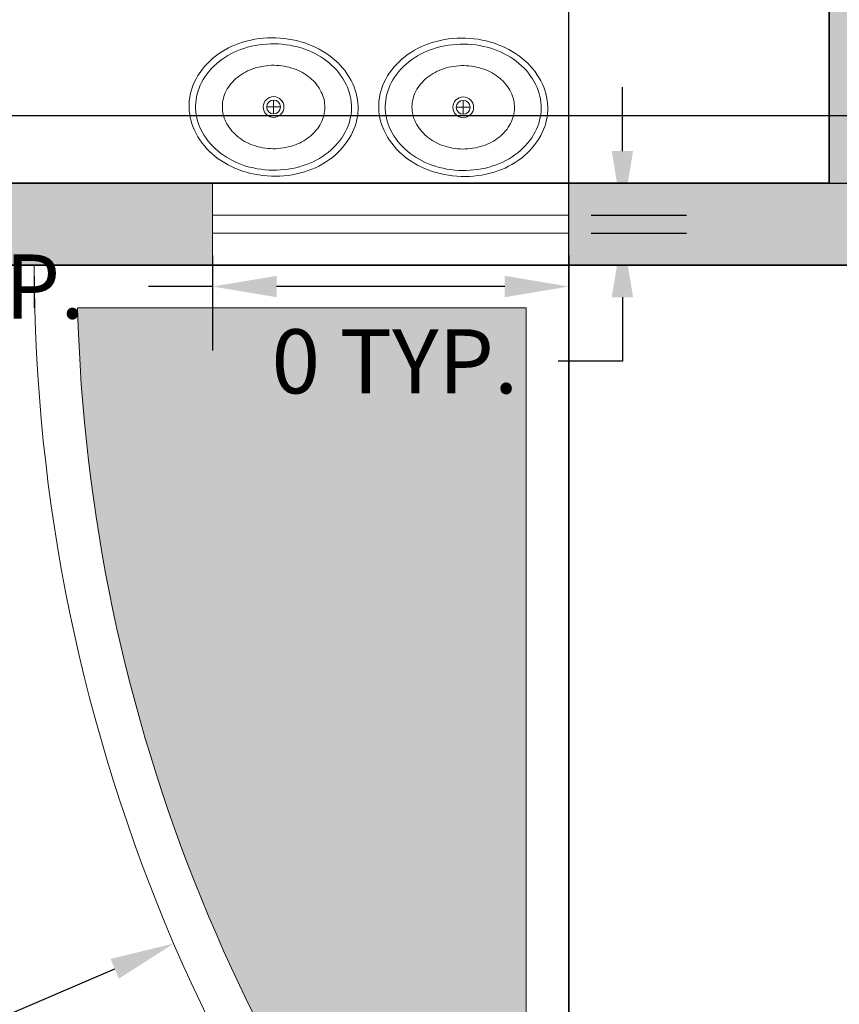
# Model space of a CAD drawing. Units: metres. Extents: x 4298.5 to 4325.2, y 2075 to 2095.8.
# Tile 11 of 35: x 4307.6 to 4309.9, y 2077.8 to 2080.5. Entities that reach past the tile are written whole.
import ezdxf

# ---------------------------------------------------------------- set-up
doc = ezdxf.new("R2010")
doc.units = ezdxf.units.M
for name, color, linetype, lineweight in [('A-ANNO-DIMS', 2, 'Continuous', 18), ('A-FLOR-FIXT', 15, 'Continuous', 18), ('A-FLOR-STRS', 7, 'Continuous', 25), ('A-GLAZ', 4, 'Continuous', 18), ('A-WALL', 7, 'Continuous', 35), ('A-WALL-PATT', 252, 'Continuous', 13), ('L-PLNT-BEDS', 94, 'Continuous', 18), ('L-PLNT-BEDS-PATT', 252, 'Continuous', 13)]:
    doc.layers.add(name, color=color, linetype=linetype, lineweight=lineweight)
doc.styles.get("Standard").update_dxf_attribs({"font": 'arial.ttf'})
doc.dimstyles.get("Standard").update_dxf_attribs({"dimtxt": 0.18, "dimasz": 0.18, "dimexe": 0.18, "dimexo": 0.0625, "dimgap": 0.09, "dimtad": 0, "dimtih": 1, "dimtoh": 1, "dimdec": 4, "dimzin": 0, "dimdsep": 46, "dimtxsty": 'Standard', "dimcen": 0.09, "dimadec": 0, "dimazin": 0, "dimtfac": 1, "dimtdec": 4, "dimtofl": 0, "dimtmove": 0, "dimatfit": 3, "dimfxl": 1, "dimtolj": 1, "dimtzin": 0, "dimarcsym": 0})

# ---------------------------------------------------------------- blocks, each defined once
blk = doc.blocks.new('Sink - Oval top')
for p, q in [((-1, 0), (1, 0)), ((0, 1), (0, -1))]:
    blk.add_line(p, q)
for points in [[(-12.23, 0.39, 0.117634), (-11.46, -3.36, 0.104469), (-8.88, -6.8, 0.090016), (-5.08, -9.07, 0.08192), (-0.32, -10.02, 0.08192), (4.49, -9.38, 0.090016), (8.42, -7.36, 0.104469), (11.22, -4.09, 0.117634), (12.23, -0.39, 0.117634), (11.46, 3.36, 0.104469), (8.88, 6.8, 0.090016), (5.08, 9.07, 0.08192), (0.32, 10.02, 0.08192), (-4.49, 9.38, 0.090016), (-8.42, 7.36, 0.104469), (-11.22, 4.09, 0.117634)], [(-11.29, 0.16, 0.118622), (-10.52, -3.25, 0.104678), (-8.07, -6.36, 0.089562), (-4.54, -8.37, 0.081185), (-0.13, -9.15, 0.081185), (4.3, -8.49, 0.089562), (7.89, -6.58, 0.104678), (10.42, -3.55, 0.118622), (11.29, -0.16, 0.118622), (10.52, 3.25, 0.104678), (8.07, 6.36, 0.089562), (4.54, 8.37, 0.081185), (0.13, 9.15, 0.081185), (-4.3, 8.49, 0.089562), (-7.89, 6.58, 0.104678), (-10.42, 3.55, 0.118622)], [(-7.42, 0.08, 0.118283), (-6.91, -2.17, 0.104607), (-5.29, -4.21, 0.089718), (-2.97, -5.53, 0.081436), (-0.07, -6.04, 0.081436), (2.84, -5.59, 0.089718), (5.2, -4.33, 0.104607), (6.86, -2.32, 0.118283), (7.42, -0.08, 0.118283), (6.91, 2.17, 0.104607), (5.29, 4.21, 0.089718), (2.97, 5.53, 0.081436), (0.07, 6.04, 0.081436), (-2.84, 5.59, 0.089718), (-5.2, 4.33, 0.104607), (-6.86, 2.32, 0.118283)]]:
    blk.add_lwpolyline(points, format="xyb", close=True)
for radius in [1.5, 1]:
    blk.add_circle((0, 0), radius)
blk = doc.blocks.new('WIN-1000-GLASS')
for p, q in [((1, 0.05), (0, 0.05)), ((1, 0), (0, 0))]:
    blk.add_line(p, q)
blk = doc.blocks.new('*D23')
at = {"layer": 'A-ANNO-DIMS', "color": 0, "lineweight": -2, "transparency": 16777216}
for p, q in [((4308.1606, 2079.8556), (4308.1606, 2079.5881)), ((4309.1606, 2079.8556), (4309.1606, 2079.5881)), ((4308.1606, 2079.7681), (4307.9806, 2079.7681)), ((4308.9806, 2079.7681), (4308.3406, 2079.7681))]:
    blk.add_line(p, q, dxfattribs=at)
at = {"layer": 'A-ANNO-DIMS', "color": 0, "transparency": 16777216}
for points in [[(4308.3406, 2079.7981), (4308.3406, 2079.7381), (4308.1606, 2079.7681)], [(4308.9806, 2079.7981), (4308.9806, 2079.7381), (4309.1606, 2079.7681)]]:
    blk.add_solid(points, dxfattribs=at)
at = {"layer": 'Defpoints', "color": 0, "transparency": 16777216}
for p in [(4308.1606, 2079.9181), (4309.1606, 2079.9181), (4308.1606, 2079.7681)]:
    blk.add_point(p, dxfattribs=at)
at = {"layer": 'A-ANNO-DIMS', "color": 0, "transparency": 16777216, "insert": (4306.7086, 2079.7681), "char_height": 0.18, "attachment_point": 5}
blk.add_mtext('\\A1;WINDOW W1 1 TYP.', dxfattribs=at)
blk = doc.blocks.new('*D24')
at = {"layer": 'A-ANNO-DIMS', "color": 0, "lineweight": -2, "transparency": 16777216}
for p, q in [((4309.3106, 2080.1481), (4309.3106, 2080.3281)), ((4309.2231, 2079.9681), (4309.4906, 2079.9681)), ((4309.2231, 2079.9181), (4309.4906, 2079.9181)), ((4309.3106, 2079.7381), (4309.3106, 2079.5581)), ((4309.3106, 2079.5581), (4309.1306, 2079.5581))]:
    blk.add_line(p, q, dxfattribs=at)
at = {"layer": 'A-ANNO-DIMS', "color": 0, "transparency": 16777216}
for points in [[(4309.2806, 2080.1481), (4309.3406, 2080.1481), (4309.3106, 2079.9681)], [(4309.2806, 2079.7381), (4309.3406, 2079.7381), (4309.3106, 2079.9181)]]:
    blk.add_solid(points, dxfattribs=at)
at = {"layer": 'Defpoints', "color": 0, "transparency": 16777216}
for p in [(4309.1606, 2079.9681), (4309.1606, 2079.9181), (4309.3106, 2079.9181)]:
    blk.add_point(p, dxfattribs=at)
at = {"layer": 'A-ANNO-DIMS', "color": 0, "transparency": 16777216, "insert": (4308.6724, 2079.5581), "char_height": 0.18, "attachment_point": 5}
blk.add_mtext('\\A1;0 TYP.', dxfattribs=at)
blk = doc.blocks.new('*D47')
at = {"layer": 'A-ANNO-DIMS', "color": 0, "lineweight": -2, "transparency": 16777216}
for p, q in [((4300.4306, 2084.4956), (4300.4306, 2074.9896)), ((4322.8106, 2084.4956), (4322.8106, 2074.9896)), ((4300.6106, 2075.1696), (4311.2252, 2075.1696)), ((4322.6306, 2075.1696), (4312.016, 2075.1696))]:
    blk.add_line(p, q, dxfattribs=at)
at = {"layer": 'A-ANNO-DIMS', "color": 0, "transparency": 16777216}
for points in [[(4300.6106, 2075.1996), (4300.6106, 2075.1396), (4300.4306, 2075.1696)], [(4322.6306, 2075.1996), (4322.6306, 2075.1396), (4322.8106, 2075.1696)]]:
    blk.add_solid(points, dxfattribs=at)
at = {"layer": 'Defpoints', "color": 0, "transparency": 16777216}
for p in [(4300.4306, 2084.5581), (4322.8106, 2084.5581), (4322.8106, 2075.1696)]:
    blk.add_point(p, dxfattribs=at)
at = {"layer": 'A-ANNO-DIMS', "color": 0, "transparency": 16777216, "insert": (4311.6206, 2075.1696), "char_height": 0.18, "attachment_point": 5}
blk.add_mtext('\\A1;22.38', dxfattribs=at)
blk = doc.blocks.new('*D53')
at = {"layer": 'A-ANNO-DIMS', "color": 0, "lineweight": -2, "transparency": 16777216}
for p, q in [((4309.1606, 2076.3906), (4309.1606, 2095.8166)), ((4316.8106, 2076.3906), (4316.8106, 2095.8166)), ((4309.3406, 2095.6366), (4312.6619, 2095.6366)), ((4316.6306, 2095.6366), (4313.3093, 2095.6366))]:
    blk.add_line(p, q, dxfattribs=at)
at = {"layer": 'A-ANNO-DIMS', "color": 0, "transparency": 16777216}
for points in [[(4309.3406, 2095.6666), (4309.3406, 2095.6066), (4309.1606, 2095.6366)], [(4316.6306, 2095.6666), (4316.6306, 2095.6066), (4316.8106, 2095.6366)]]:
    blk.add_solid(points, dxfattribs=at)
at = {"layer": 'Defpoints', "color": 0, "transparency": 16777216}
for p in [(4316.8106, 2095.6366), (4309.1606, 2076.3281), (4316.8106, 2076.3281)]:
    blk.add_point(p, dxfattribs=at)
at = {"layer": 'A-ANNO-DIMS', "color": 0, "transparency": 16777216, "insert": (4312.9856, 2095.6366), "char_height": 0.18, "attachment_point": 5}
blk.add_mtext('\\A1;7.65', dxfattribs=at)
blk = doc.blocks.new('*D54')
at = {"layer": 'A-ANNO-DIMS', "color": 0, "lineweight": -2, "transparency": 16777216}
for p, q in [((4305.5981, 2079.8281), (4299.0921, 2079.8281)), ((4299.2721, 2079.6481), (4299.2721, 2078.26)), ((4299.2721, 2076.5081), (4299.2721, 2077.8961)), ((4309.0981, 2076.3281), (4299.0921, 2076.3281))]:
    blk.add_line(p, q, dxfattribs=at)
at = {"layer": 'A-ANNO-DIMS', "color": 0, "transparency": 16777216}
for points in [[(4299.2421, 2079.6481), (4299.3021, 2079.6481), (4299.2721, 2079.8281)], [(4299.2421, 2076.5081), (4299.3021, 2076.5081), (4299.2721, 2076.3281)]]:
    blk.add_solid(points, dxfattribs=at)
at = {"layer": 'Defpoints', "color": 0, "transparency": 16777216}
for p in [(4305.6606, 2079.8281), (4299.2721, 2076.3281), (4309.1606, 2076.3281)]:
    blk.add_point(p, dxfattribs=at)
at = {"layer": 'A-ANNO-DIMS', "color": 0, "transparency": 16777216, "insert": (4299.2721, 2078.0781), "char_height": 0.18, "attachment_point": 5}
blk.add_mtext('\\A1;3.5', dxfattribs=at)
blk = doc.blocks.new('*D60')
at = {"layer": 'A-ANNO-DIMS', "color": 0, "lineweight": -2, "transparency": 16777216}
for p, q in [((4305.9531, 2081.9381), (4324.7671, 2081.9381)), ((4324.5871, 2081.7581), (4324.5871, 2081.18)), ((4324.5871, 2080.2381), (4324.5871, 2080.8162)), ((4305.9531, 2080.0581), (4324.7671, 2080.0581))]:
    blk.add_line(p, q, dxfattribs=at)
at = {"layer": 'A-ANNO-DIMS', "color": 0, "transparency": 16777216}
for points in [[(4324.5571, 2081.7581), (4324.6171, 2081.7581), (4324.5871, 2081.9381)], [(4324.5571, 2080.2381), (4324.6171, 2080.2381), (4324.5871, 2080.0581)]]:
    blk.add_solid(points, dxfattribs=at)
at = {"layer": 'Defpoints', "color": 0, "transparency": 16777216}
for p in [(4305.8906, 2081.9381), (4324.5871, 2081.9381), (4305.8906, 2080.0581)]:
    blk.add_point(p, dxfattribs=at)
at = {"layer": 'A-ANNO-DIMS', "color": 0, "transparency": 16777216, "insert": (4324.5871, 2080.9981), "char_height": 0.18, "attachment_point": 5}
blk.add_mtext('\\A1;1.88', dxfattribs=at)
blk = doc.blocks.new('*D64')
at = {"layer": 'A-ANNO-DIMS', "color": 0, "lineweight": -2, "transparency": 16777216}
for p, q in [((4312.1097, 2081.1221), (4299.0921, 2081.1221)), ((4299.2721, 2080.9421), (4299.2721, 2080.427)), ((4312.1097, 2080.247), (4299.0921, 2080.247)), ((4299.2721, 2080.247), (4299.2721, 2080.067)), ((4299.2721, 2080.067), (4299.0921, 2080.067))]:
    blk.add_line(p, q, dxfattribs=at)
at = {"layer": 'A-ANNO-DIMS', "color": 0, "transparency": 16777216}
for points in [[(4299.2421, 2080.9421), (4299.3021, 2080.9421), (4299.2721, 2081.1221)], [(4299.2421, 2080.427), (4299.3021, 2080.427), (4299.2721, 2080.247)]]:
    blk.add_solid(points, dxfattribs=at)
at = {"layer": 'Defpoints', "color": 0, "transparency": 16777216}
for p in [(4312.1722, 2081.1221), (4299.2721, 2080.247), (4312.1722, 2080.247)]:
    blk.add_point(p, dxfattribs=at)
at = {"layer": 'A-ANNO-DIMS', "color": 0, "transparency": 16777216, "insert": (4298.7681, 2080.067), "char_height": 0.18, "attachment_point": 5}
blk.add_mtext('\\A1;0.88', dxfattribs=at)
blk = doc.blocks.new('*D78')
at = {"layer": 'A-ANNO-DIMS', "color": 0, "lineweight": -2, "transparency": 16777216}
for p, q in [((4312.4969, 2079.7393), (4312.4969, 2079.9193)), ((4312.4069, 2079.8293), (4312.5869, 2079.8293)), ((4305.3847, 2076.7806), (4307.8863, 2077.853)), ((4305.2047, 2076.7806), (4305.3847, 2076.7806))]:
    blk.add_line(p, q, dxfattribs=at)
at = {"layer": 'A-ANNO-DIMS', "color": 0, "transparency": 16777216}
blk.add_solid([(4307.8745, 2077.8806), (4307.8981, 2077.8254), (4308.0518, 2077.9239)], dxfattribs=at)
at = {"layer": 'Defpoints', "color": 0, "transparency": 16777216}
for p in [(4312.4969, 2079.8293), (4308.0518, 2077.9239)]:
    blk.add_point(p, dxfattribs=at)
at = {"layer": 'A-ANNO-DIMS', "color": 0, "transparency": 16777216, "insert": (4304.53, 2076.7806), "char_height": 0.18, "attachment_point": 5}
blk.add_mtext('\\A1;2X R4.836', dxfattribs=at)

msp = doc.modelspace()

# ---------------------------------------------------------------- hatches: boundary and pattern name
at = {"layer": 'A-WALL-PATT'}
h = msp.add_hatch(color=256, dxfattribs=at)
h.dxf.hatch_style = 1
h.paths.add_polyline_path([(4308.7606, 2094.4781), (4308.1606, 2094.4781), (4307.4606, 2094.4781), (4307.4606, 2094.2481), (4308.2706, 2094.2481), (4308.2706, 2094.1281), (4308.3906, 2094.1281), (4308.3906, 2094.2481), (4308.7606, 2094.2481)])
h.paths.add_polyline_path([(4310.1206, 2094.4781), (4309.5206, 2094.4781), (4309.5206, 2094.2481), (4309.8906, 2094.2481), (4309.8906, 2092.2481), (4308.3906, 2092.2481), (4308.3906, 2093.4281), (4308.2706, 2093.4281), (4308.2706, 2092.0181), (4309.8906, 2092.0181), (4309.8906, 2087.0181), (4309.7706, 2087.0181), (4309.7706, 2086.7881), (4309.8906, 2086.7881), (4311.9406, 2086.7881), (4311.9406, 2087.0181), (4310.1206, 2087.0181), (4310.1206, 2089.0181), (4310.2406, 2089.0181), (4310.2406, 2089.1381), (4310.1206, 2089.1381), (4310.1206, 2092.0181), (4310.3078, 2092.0181), (4310.3078, 2092.2481), (4310.1206, 2092.2481)])
h.paths.add_polyline_path([(4311.7406, 2092.2481), (4311.0678, 2092.2481), (4311.0678, 2092.0181), (4311.7406, 2092.0181)], flags=17)
h.paths.add_polyline_path([(4313.1733, 2092.2481), (4312.5006, 2092.2481), (4312.5006, 2092.0181), (4313.1733, 2092.0181)])
h.paths.add_polyline_path([(4314.5378, 2092.2481), (4314.1206, 2092.2481), (4313.9333, 2092.2481), (4313.9333, 2092.0181), (4314.1206, 2092.0181), (4314.1206, 2087.0181), (4314.0006, 2087.0181), (4314.0006, 2086.7881), (4314.1206, 2086.7881), (4315.5718, 2086.7881), (4315.5718, 2087.0181), (4314.3506, 2087.0181), (4314.3506, 2092.0181), (4314.5378, 2092.0181)])
h.paths.add_polyline_path([(4315.9706, 2092.2481), (4315.2978, 2092.2481), (4315.2978, 2092.0181), (4315.9706, 2092.0181)])
h.paths.add_polyline_path([(4317.4033, 2092.2481), (4316.7306, 2092.2481), (4316.7306, 2092.0181), (4317.4033, 2092.0181)])
h.paths.add_polyline_path([(4318.9506, 2092.2481), (4318.3506, 2092.2481), (4318.1633, 2092.2481), (4318.1633, 2092.0181), (4318.3506, 2092.0181), (4318.3506, 2091.8981), (4318.5806, 2091.8981), (4318.5806, 2092.0181), (4318.9506, 2092.0181)])
h.paths.add_polyline_path([(4321.0106, 2092.2481), (4319.7106, 2092.2481), (4319.7106, 2092.0181), (4320.0806, 2092.0181), (4320.0806, 2090.0181), (4318.5806, 2090.0181), (4318.5806, 2091.1981), (4318.3506, 2091.1981), (4318.3506, 2090.0181), (4318.3506, 2087.0181), (4318.2306, 2087.0181), (4318.2306, 2086.7881), (4318.3506, 2086.7881), (4318.3506, 2086.3081), (4318.5806, 2086.3081), (4318.5806, 2089.7881), (4321.7806, 2089.7881), (4321.7806, 2090.0181), (4320.2006, 2090.0181), (4320.2006, 2092.0181), (4321.0106, 2092.0181)])
h.paths.add_polyline_path([(4322.8106, 2092.2481), (4321.7706, 2092.2481), (4321.7706, 2092.0181), (4322.5806, 2092.0181), (4322.5806, 2091.2831), (4322.8106, 2091.2831)])
h.paths.add_polyline_path([(4322.8106, 2090.5231), (4322.5806, 2090.5231), (4322.5806, 2089.7881), (4322.5806, 2089.5254), (4322.8106, 2089.5254), (4322.8106, 2090.0181)])
h.paths.add_polyline_path([(4322.8106, 2088.7654), (4322.5806, 2088.7654), (4322.5806, 2087.6681), (4322.8106, 2087.6681)])
h.paths.add_polyline_path([(4322.8106, 2086.9081), (4322.5806, 2086.9081), (4322.5806, 2085.8107), (4322.8106, 2085.8107)])
h.paths.add_polyline_path([(4322.8106, 2085.0507), (4322.5806, 2085.0507), (4322.5806, 2084.7881), (4318.5806, 2084.7881), (4318.5806, 2085.0581), (4318.5806, 2085.4081), (4318.3506, 2085.4081), (4318.3506, 2084.5581), (4318.3506, 2080.8581), (4318.4706, 2080.8581), (4318.4706, 2082.3281), (4319.2606, 2082.3281), (4319.2606, 2082.5581), (4318.5806, 2082.5581), (4318.5806, 2084.5581), (4320.0806, 2084.5581), (4320.0806, 2083.9381), (4320.3106, 2083.9381), (4320.3106, 2084.5581), (4322.8106, 2084.5581)])
h.paths.add_polyline_path([(4320.3106, 2083.1781), (4320.0806, 2083.1781), (4320.0806, 2082.5581), (4319.9606, 2082.5581), (4319.9606, 2082.3281), (4320.0806, 2082.3281), (4320.0806, 2081.5731), (4320.3106, 2081.5731)], flags=17)
h.paths.add_polyline_path([(4320.3106, 2080.8131), (4320.0806, 2080.8131), (4320.0806, 2080.0581), (4318.4286, 2080.0581), (4318.4286, 2079.8281), (4320.3106, 2079.8281)])
h.paths.add_polyline_path([(4317.3506, 2085.2881), (4316.5718, 2085.2881), (4316.5718, 2085.0581), (4317.3506, 2085.0581)])
h.paths.add_polyline_path([(4315.5718, 2085.2881), (4314.8434, 2085.2881), (4314.8434, 2085.0581), (4315.5718, 2085.0581)])
h.paths.add_polyline_path([(4313.8434, 2085.2881), (4312.9406, 2085.2881), (4312.9406, 2085.0581), (4313.8434, 2085.0581)])
h.paths.add_polyline_path([(4311.9406, 2085.2881), (4311.4406, 2085.2881), (4311.4406, 2085.0581), (4311.9406, 2085.0581)])
h.paths.add_polyline_path([(4317.3306, 2087.0181), (4316.5718, 2087.0181), (4316.5718, 2086.7881), (4317.3306, 2086.7881)])
h.paths.add_polyline_path([(4313.1006, 2089.1381), (4311.1406, 2089.1381), (4311.1406, 2089.0181), (4312.9806, 2089.0181), (4312.9806, 2087.0181), (4312.9406, 2087.0181), (4312.9406, 2086.7881), (4313.1006, 2086.7881), (4313.1006, 2087.0181)])
h.paths.add_polyline_path([(4307.5515, 2087.0181), (4305.8906, 2087.0181), (4305.8906, 2092.2481), (4305.8906, 2094.2481), (4306.7006, 2094.2481), (4306.7006, 2094.4781), (4305.6606, 2094.4781), (4305.6606, 2092.2481), (4305.2906, 2092.2481), (4305.2906, 2092.0181), (4305.6606, 2092.0181), (4305.6606, 2090.0181), (4304.1606, 2090.0181), (4304.1606, 2091.1981), (4304.0406, 2091.1981), (4304.0406, 2089.9081), (4301.5606, 2089.9081), (4301.5606, 2089.7881), (4304.0406, 2089.7881), (4305.6606, 2089.7881), (4305.6606, 2086.6381), (4305.8906, 2086.6381), (4305.8906, 2086.7881), (4307.5515, 2086.7881)])
h.paths.add_polyline_path([(4307.5515, 2085.2881), (4305.8906, 2085.2881), (4305.8906, 2085.4381), (4305.6606, 2085.4381), (4305.6606, 2084.7881), (4305.2906, 2084.7881), (4305.2906, 2084.5581), (4305.6606, 2084.5581), (4305.6606, 2084.02), (4305.8906, 2084.02), (4305.8906, 2084.5581), (4305.8906, 2085.0581), (4307.5515, 2085.0581)])
h.paths.add_polyline_path([(4310.2406, 2085.2881), (4308.5515, 2085.2881), (4308.5515, 2085.0581), (4310.2406, 2085.0581)])
h.paths.add_polyline_path([(4317.4286, 2080.0581), (4316.5718, 2080.0581), (4316.5718, 2079.8281), (4317.4286, 2079.8281)])
h.paths.add_polyline_path([(4315.5718, 2080.0581), (4314.8434, 2080.0581), (4314.8434, 2079.8281), (4315.5718, 2079.8281)])
h.paths.add_polyline_path([(4313.8434, 2080.0581), (4312.9406, 2080.0581), (4312.9406, 2079.8281), (4313.8434, 2079.8281)])
h.paths.add_polyline_path([(4311.9406, 2080.0581), (4311.4406, 2080.0581), (4311.4406, 2079.8281), (4311.9406, 2079.8281)])
h.paths.add_polyline_path([(4310.2406, 2080.0581), (4310.1206, 2080.0581), (4310.1206, 2084.0381), (4309.8906, 2084.0381), (4309.8906, 2080.0581), (4309.1606, 2080.0581), (4309.1606, 2079.8281), (4310.2406, 2079.8281)])
h.paths.add_polyline_path([(4308.1606, 2080.0581), (4307.5106, 2080.0581), (4307.5106, 2080.1781), (4307.3906, 2080.1781), (4307.3906, 2080.0581), (4305.8906, 2080.0581), (4305.8906, 2080.567), (4305.6606, 2080.567), (4305.6606, 2079.8281), (4308.1606, 2079.8281)])
h.paths.add_polyline_path([(4307.5106, 2081.9381), (4309.0906, 2081.9381), (4309.0906, 2082.0581), (4305.8906, 2082.0581), (4305.8906, 2083.26), (4305.6606, 2083.26), (4305.6606, 2081.327), (4305.8906, 2081.327), (4305.8906, 2081.9381), (4307.3906, 2081.9381), (4307.3906, 2080.8781), (4307.5106, 2080.8781)])
h.paths.add_polyline_path([(4304.5306, 2084.7881), (4302.7306, 2084.7881), (4302.7306, 2084.5581), (4304.5306, 2084.5581)])
h.paths.add_polyline_path([(4301.9706, 2084.7881), (4300.6606, 2084.7881), (4300.6606, 2085.0249), (4300.4306, 2085.0249), (4300.4306, 2084.5581), (4301.9706, 2084.5581)])
h.paths.add_polyline_path([(4300.6606, 2086.8843), (4300.4306, 2086.8843), (4300.4306, 2085.7849), (4300.6606, 2085.7849)])
h.paths.add_polyline_path([(4300.6606, 2089.1618), (4300.4306, 2089.1618), (4300.4306, 2087.6443), (4300.6606, 2087.6443)])
h.paths.add_polyline_path([(4300.6606, 2091.0212), (4300.4306, 2091.0212), (4300.4306, 2089.9218), (4300.6606, 2089.9218)])
h.paths.add_polyline_path([(4300.6606, 2092.0181), (4301.9706, 2092.0181), (4301.9706, 2092.2481), (4300.4306, 2092.2481), (4300.4306, 2091.7812), (4300.6606, 2091.7812)])
h.paths.add_polyline_path([(4304.5306, 2092.2481), (4302.7306, 2092.2481), (4302.7306, 2092.0181), (4304.0406, 2092.0181), (4304.0406, 2091.8981), (4304.1606, 2091.8981), (4304.1606, 2092.0181), (4304.5306, 2092.0181)], flags=17)
at = {"layer": 'L-PLNT-BEDS-PATT'}
h = msp.add_hatch(dxfattribs=at)
h.set_pattern_fill('TRIANG', color=256, scale=0.02)
h.paths.add_polyline_path([(4309.0406, 2079.7081), (4307.7821, 2079.7081, 0.182638), (4309.0406, 2076.6204)])
h.paths.add_polyline_path([(4318.189, 2079.7081), (4316.9306, 2079.7081), (4316.9306, 2076.6204, 0.182638)])

# ---------------------------------------------------------------- linework, layer by layer
at = {"layer": 'A-FLOR-STRS'}
msp.add_line((4309.1606, 2079.8281), (4309.1606, 2076.3281), dxfattribs=at)
at = {"layer": 'A-GLAZ'}
for p, q in [((4308.1606, 2079.8281), (4308.1606, 2080.0581)), ((4309.1606, 2079.8281), (4309.1606, 2080.0581))]:
    msp.add_line(p, q, dxfattribs=at)
at = {"layer": 'A-WALL'}
for p, q in [((4309.8906, 2084.0381), (4309.8906, 2080.0581)), ((4307.5106, 2080.0581), (4309.8906, 2080.0581)), ((4310.2406, 2079.8281), (4305.6606, 2079.8281))]:
    msp.add_line(p, q, dxfattribs=at)
at = {"layer": 'L-PLNT-BEDS'}
for p, q in [((4307.6606, 2079.8281), (4307.6606, 2079.7081)), ((4307.6621, 2079.7081), (4307.6606, 2079.7081)), ((4309.0406, 2079.7081), (4307.7821, 2079.7081)), ((4309.0406, 2079.7081), (4309.0406, 2076.6204))]:
    msp.add_line(p, q, dxfattribs=at)
for radius, start, end in [(4.8363, 180.0152, 226.382), (4.7163, 180.0152, 180.0156), (4.7163, 181.4735, 222.8748)]:
    msp.add_arc((4312.4969, 2079.8293), radius, start, end, dxfattribs=at)

# ---------------------------------------------------------------- block references
at = {"layer": 'A-FLOR-FIXT', "xscale": 0.0193818050953029, "yscale": 0.0193818050953029, "zscale": 0.0193818050953029}
for p in [(4308.332, 2080.272), (4308.8641, 2080.2711)]:
    msp.add_blockref('Sink - Oval top', p, dxfattribs=at)
at = {"layer": 'A-GLAZ', "rotation": 180}
msp.add_blockref('WIN-1000-GLASS', (4309.1606, 2079.9681), dxfattribs=at)

# ---------------------------------------------------------------- dimensions: what is measured, and where the dimension line sits
at = {"layer": 'A-ANNO-DIMS'}
for base, p1, p2, picture, middle in [((4316.8106, 2095.6366), (4309.1606, 2076.3281), (4316.8106, 2076.3281), '*D53', (4312.9856, 2095.6366)), ((4322.8106, 2075.1696), (4300.4306, 2084.5581), (4322.8106, 2084.5581), '*D47', (4311.6206, 2075.1696))]:
    dim = msp.add_linear_dim(base=base, p1=p1, p2=p2, dimstyle='Standard', override={"dimdec": 2, "dimlfac": 1, "dimrnd": 0, "dimzin": 0, "dimdsep": 46, "dimlunit": 2}, dxfattribs=at)
    dim.commit()
    dim.dimension.update_dxf_attribs({"geometry": picture, "text_midpoint": middle})
for base, p1, p2, override, picture, middle in [((4324.5871, 2081.9381), (4305.8906, 2080.0581), (4305.8906, 2081.9381), {"dimdec": 2, "dimlfac": 1, "dimrnd": 0, "dimzin": 0, "dimdsep": 46, "dimlunit": 2}, '*D60', (4324.5871, 2080.9981)), ((4299.2721, 2080.247), (4312.1722, 2081.1221), (4312.1722, 2080.247), {"dimdec": 2, "dimlfac": 1, "dimrnd": 0, "dimzin": 0, "dimdsep": 46, "dimlunit": 2}, '*D64', (4298.7681, 2080.067)), ((4299.2721, 2076.3281), (4305.6606, 2079.8281), (4309.1606, 2076.3281), {"dimdec": 1, "dimlfac": 1, "dimrnd": 0, "dimzin": 0, "dimdsep": 46, "dimlunit": 2}, '*D54', (4299.2721, 2078.0781))]:
    dim = msp.add_linear_dim(base=base, p1=p1, p2=p2, angle=90, dimstyle='Standard', override=override, dxfattribs=at)
    dim.commit()
    dim.dimension.update_dxf_attribs({"geometry": picture, "text_midpoint": middle})
for base, p1, p2, angle, text, picture, middle in [((4308.1606, 2079.7681), (4309.1606, 2079.9181), (4308.1606, 2079.9181), 180, 'WINDOW W1 <> TYP.', '*D23', (4306.7086, 2079.7681)), ((4309.3106, 2079.9181), (4309.1606, 2079.9681), (4309.1606, 2079.9181), 270, '<> TYP.', '*D24', (4308.6724, 2079.5581))]:
    dim = msp.add_linear_dim(base=base, p1=p1, p2=p2, angle=angle, text=text, dimstyle='Standard', override={"dimdec": 0, "dimlfac": 1, "dimrnd": 0, "dimzin": 0, "dimdsep": 46, "dimlunit": 2}, dxfattribs=at)
    dim.commit()
    dim.dimension.update_dxf_attribs({"geometry": picture, "text_midpoint": middle})
dim = msp.add_radius_dim(center=(4312.4969, 2079.8293), mpoint=(4308.0518, 2077.9239), text='2X <>', dimstyle='Standard', override={"dimdec": 3, "dimlfac": 1, "dimrnd": 0, "dimzin": 0, "dimdsep": 46, "dimlunit": 2}, dxfattribs=at)
dim.commit()
dim.dimension.update_dxf_attribs({"geometry": '*D78', "text_midpoint": (4304.53, 2076.7806), "dimtype": 164})

doc.saveas('drawing.dxf')
